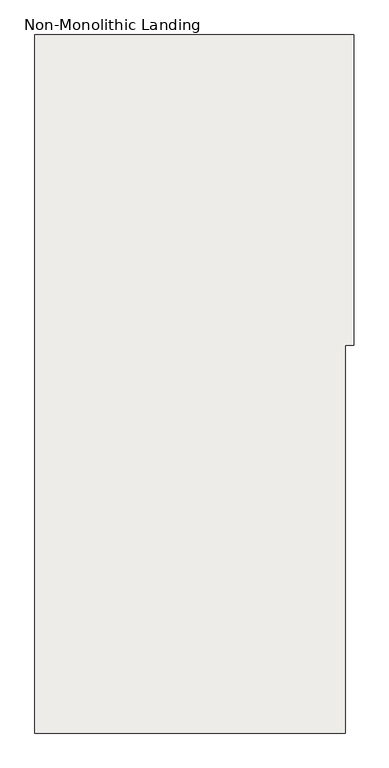
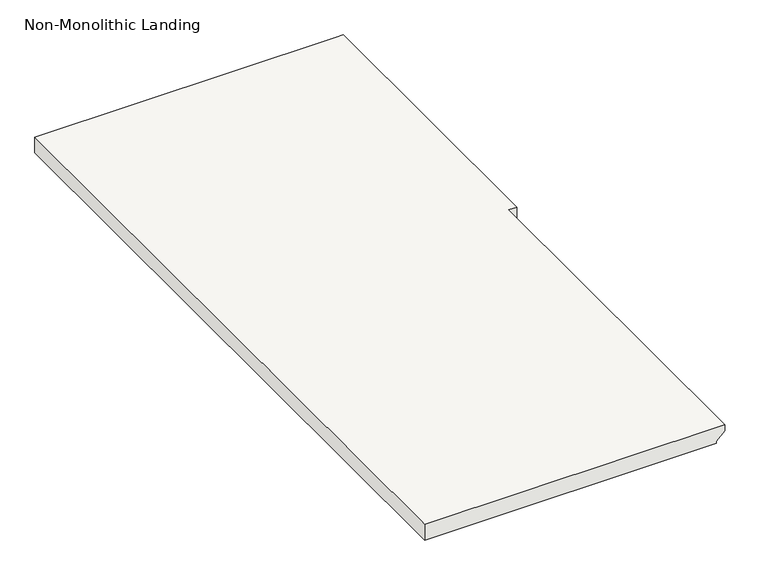
"""IFC4 building model written with IfcOpenShell, lengths in millimetres: slab geometry, Non-Monolithic Landing."""

from ifc_helpers import new_model, si_unit, origin, place, context, project, spatial, faceted_brep, source, transform, mapped, element, save


def non_monolithic_landing_1e1f2eae(model_context):
    return source(origin(), model_context, "Body", "Brep", [
        faceted_brep([(-14575.9777023, -354.9320925, 1640.4166667), (-14601.3777023, -354.9320925, 1615.0166667), (-14601.3777023, 559.4679075, 1615.0166667), (-14575.9777023, 559.4679075, 1640.4166667), (-14575.9777023, 788.0679075, 1659.4666667), (-14550.5777023, 788.0679075, 1659.4666667), (-14550.5777023, 1702.4679075, 1659.4666667), (-14575.9777023, 1702.4679075, 1659.4666667), (-15490.3777023, 1702.4679075, 1659.4666667), (-15490.3777023, -354.9320925, 1659.4666667), (-14575.9777023, -354.9320925, 1659.4666667), (-14601.3777023, 559.4679075, 1608.6666667), (-14601.3777023, -354.9320925, 1608.6666667), (-15490.3777023, -354.9320925, 1608.6666667), (-15490.3777023, 1702.4679075, 1608.6666667), (-14575.9777023, 1702.4679075, 1608.6666667), (-14550.5777023, 1702.4679075, 1608.6666667), (-14550.5777023, 788.0679075, 1608.6666667), (-14575.9777023, 788.0679075, 1608.6666667), (-14575.9777023, 559.4679075, 1608.6666667)], [[[0, 1, 2, 3]], [[4, 5, 6, 7, 8, 9, 10]], [[11, 12, 13, 14, 15, 16, 17, 18, 19]], [[12, 11, 2, 1]], [[11, 19, 3, 2]], [[4, 10, 0, 3, 19, 18]], [[5, 4, 18, 17]], [[6, 5, 17, 16]], [[7, 6, 16, 15]], [[8, 7, 15, 14]], [[9, 8, 14, 13]], [[10, 9, 13, 12, 1, 0]]]),
    ])


if __name__ == "__main__":
    model = new_model("IFC4")
    model_context = context("Model", 3, world=origin())
    ifc_project = project(units=[si_unit("LENGTHUNIT", "METRE", prefix="MILLI")], contexts=[model_context])
    site = spatial("IfcSite", under=ifc_project)
    building = spatial("IfcBuilding", under=site)
    placement = place(None, origin())
    non_monolithic_landing_shape = non_monolithic_landing_1e1f2eae(model_context)
    element("IfcSlab", 1, ObjectType="Non-Monolithic Landing", at=placement, inside=building, context=model_context, shape_type="MappedRepresentation", body=[
        mapped(non_monolithic_landing_shape, transform((0.0, 0.0, 0.0), x_axis=(1.0, 0.0, 0.0), y_axis=(0.0, 1.0, 0.0), z_axis=(0.0, 0.0, 1.0))),
    ])
    save(model, "model.ifc")
